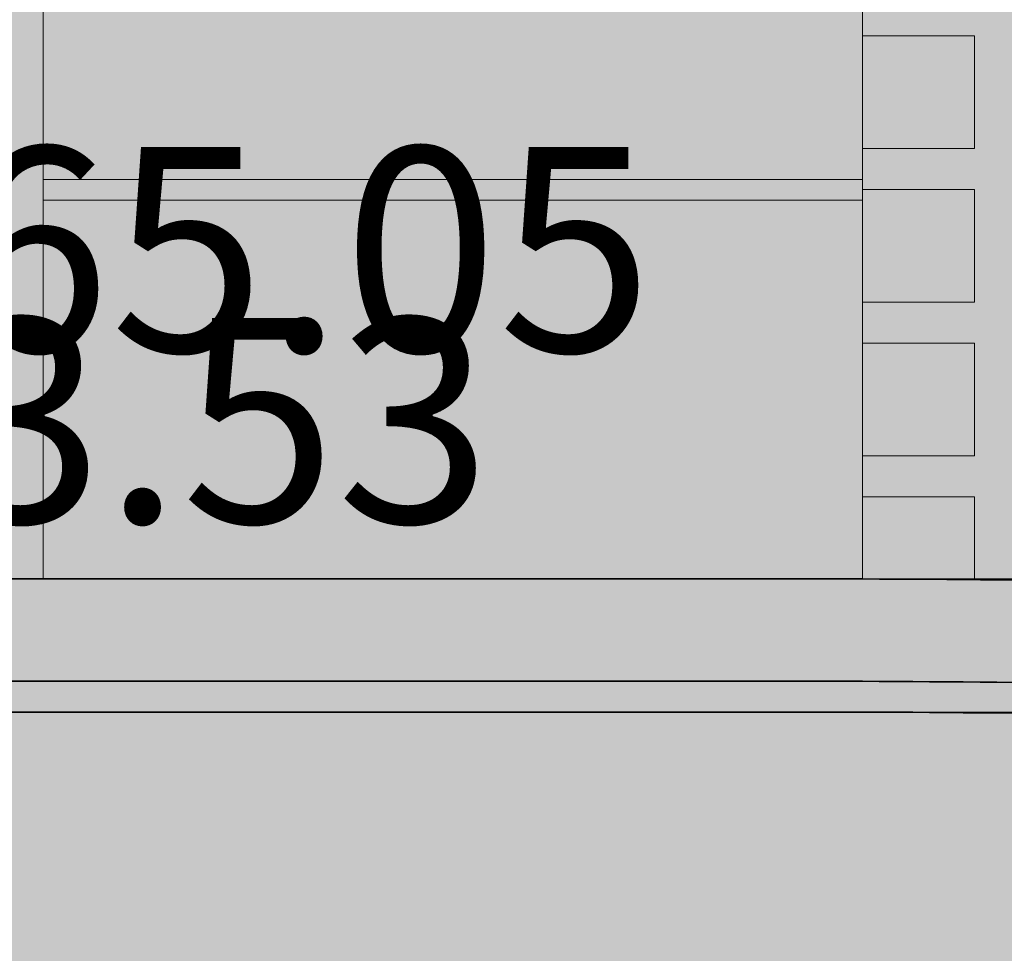
# Model space of a CAD drawing. Units: millimetres. Extents: x 130 to 1021, y 147 to 699.
# Tile 36 of 40: x 550 to 646, y 440 to 532. Entities that reach past the tile are written whole.
import ezdxf

# ---------------------------------------------------------------- set-up
doc = ezdxf.new("R2010")
doc.units = ezdxf.units.MM
doc.header["$MEASUREMENT"] = 0
for name, color, linetype, lineweight in [('A-ANNO-DIMS', 2, 'Continuous', 18), ('A-ELEV', 7, 'Continuous', 35), ('A-ELEV-PATT', 9, 'Continuous', 13), ('A-GLAZ', 4, 'Continuous', 18)]:
    doc.layers.add(name, color=color, linetype=linetype, lineweight=lineweight)
doc.styles.get("Standard").update_dxf_attribs({"font": 'arial.ttf'})
doc.dimstyles.get("Standard").update_dxf_attribs({"dimtxt": 20, "dimasz": 10, "dimexe": 10, "dimexo": 10, "dimgap": 5, "dimtad": 0, "dimtih": 1, "dimtoh": 1, "dimdec": 0, "dimzin": 0, "dimdsep": 46, "dimtxsty": 'Standard', "dimcen": 5, "dimadec": 0, "dimazin": 0, "dimtfac": 1, "dimtdec": 0, "dimtofl": 0, "dimtmove": 0, "dimatfit": 3, "dimfxl": 1, "dimtolj": 1, "dimtzin": 0, "dimarcsym": 0})

# ---------------------------------------------------------------- blocks, each defined once
blk = doc.blocks.new('*D11')
at = {"layer": 'A-ANNO-DIMS', "color": 0, "lineweight": -2, "transparency": 16777216}
for p, q in [((737.374, 648.699), (737.374, 149.739)), ((299.374, 566.947), (299.374, 149.739)), ((309.374, 159.739), (490.857, 159.739)), ((727.374, 159.739), (545.891, 159.739))]:
    blk.add_line(p, q, dxfattribs=at)
at = {"layer": 'A-ANNO-DIMS', "color": 0, "transparency": 16777216}
for points in [[(309.374, 161.406), (309.374, 158.073), (299.374, 159.739)], [(727.374, 161.406), (727.374, 158.073), (737.374, 159.739)]]:
    blk.add_solid(points, dxfattribs=at)
at = {"layer": 'Defpoints', "color": 0, "transparency": 16777216}
for p in [(737.374, 658.699), (299.374, 576.947), (737.374, 159.739)]:
    blk.add_point(p, dxfattribs=at)
at = {"layer": 'A-ANNO-DIMS', "color": 0, "transparency": 16777216, "insert": (518.374, 159.739), "char_height": 20, "attachment_point": 5}
blk.add_mtext('\\A1;438', dxfattribs=at)
blk = doc.blocks.new('*D22')
at = {"layer": 'A-ANNO-DIMS', "color": 0, "lineweight": -2, "transparency": 16777216}
for p, q in [((447.374, 656.947), (447.374, 696.247)), ((466.767, 403.947), (466.767, 696.247)), ((437.374, 686.247), (427.374, 686.247)), ((476.767, 686.247), (486.767, 686.247))]:
    blk.add_line(p, q, dxfattribs=at)
at = {"layer": 'A-ANNO-DIMS', "color": 0, "transparency": 16777216}
for points in [[(437.374, 687.914), (437.374, 684.581), (447.374, 686.247)], [(476.767, 687.914), (476.767, 684.581), (466.767, 686.247)]]:
    blk.add_solid(points, dxfattribs=at)
at = {"layer": 'Defpoints', "color": 0, "transparency": 16777216}
for p in [(466.767, 686.247), (447.374, 646.947), (466.767, 393.947)]:
    blk.add_point(p, dxfattribs=at)
at = {"layer": 'A-ANNO-DIMS', "color": 0, "transparency": 16777216, "insert": (532.34, 686.247), "char_height": 20, "attachment_point": 5}
blk.add_mtext('\\A1;19.393', dxfattribs=at)
blk = doc.blocks.new('*D23')
at = {"layer": 'A-ANNO-DIMS', "color": 0, "lineweight": -2, "transparency": 16777216}
for p, q in [((466.767, 403.947), (466.767, 696.247)), ((475.988, 209.039), (475.988, 696.247)), ((456.767, 686.247), (446.767, 686.247)), ((485.988, 686.247), (495.988, 686.247))]:
    blk.add_line(p, q, dxfattribs=at)
at = {"layer": 'A-ANNO-DIMS', "color": 0, "transparency": 16777216}
for points in [[(456.767, 687.914), (456.767, 684.581), (466.767, 686.247)], [(485.988, 687.914), (485.988, 684.581), (475.988, 686.247)]]:
    blk.add_solid(points, dxfattribs=at)
at = {"layer": 'Defpoints', "color": 0, "transparency": 16777216}
for p in [(475.988, 686.247), (466.767, 393.947), (475.988, 199.039)]:
    blk.add_point(p, dxfattribs=at)
at = {"layer": 'A-ANNO-DIMS', "color": 0, "transparency": 16777216, "insert": (534.631, 686.247), "char_height": 20, "attachment_point": 5}
blk.add_mtext('\\A1;9.222', dxfattribs=at)
blk = doc.blocks.new('*D24')
at = {"layer": 'A-ANNO-DIMS', "color": 0, "lineweight": -2, "transparency": 16777216}
for p, q in [((475.988, 209.039), (475.988, 696.247)), ((487.374, 671.947), (487.374, 696.247)), ((465.988, 686.247), (455.988, 686.247)), ((497.374, 686.247), (507.374, 686.247))]:
    blk.add_line(p, q, dxfattribs=at)
at = {"layer": 'A-ANNO-DIMS', "color": 0, "transparency": 16777216}
for points in [[(465.988, 687.914), (465.988, 684.581), (475.988, 686.247)], [(497.374, 687.914), (497.374, 684.581), (487.374, 686.247)]]:
    blk.add_solid(points, dxfattribs=at)
at = {"layer": 'Defpoints', "color": 0, "transparency": 16777216}
for p in [(487.374, 686.247), (487.374, 661.947), (475.988, 199.039)]:
    blk.add_point(p, dxfattribs=at)
at = {"layer": 'A-ANNO-DIMS', "color": 0, "transparency": 16777216, "insert": (553.022, 686.247), "char_height": 20, "attachment_point": 5}
blk.add_mtext('\\A1;11.385', dxfattribs=at)
blk = doc.blocks.new('*D25')
at = {"layer": 'A-ANNO-DIMS', "color": 0, "lineweight": -2, "transparency": 16777216}
for p, q in [((487.374, 671.947), (487.374, 696.247)), ((494.102, 506.908), (494.102, 696.247)), ((477.374, 686.247), (467.374, 686.247)), ((504.102, 686.247), (514.102, 686.247))]:
    blk.add_line(p, q, dxfattribs=at)
at = {"layer": 'A-ANNO-DIMS', "color": 0, "transparency": 16777216}
for points in [[(477.374, 687.914), (477.374, 684.581), (487.374, 686.247)], [(504.102, 687.914), (504.102, 684.581), (494.102, 686.247)]]:
    blk.add_solid(points, dxfattribs=at)
at = {"layer": 'Defpoints', "color": 0, "transparency": 16777216}
for p in [(494.102, 686.247), (487.374, 661.947), (494.102, 496.908)]:
    blk.add_point(p, dxfattribs=at)
at = {"layer": 'A-ANNO-DIMS', "color": 0, "transparency": 16777216, "insert": (552.922, 686.247), "char_height": 20, "attachment_point": 5}
blk.add_mtext('\\A1;6.728', dxfattribs=at)
blk = doc.blocks.new('*D26')
at = {"layer": 'A-ANNO-DIMS', "color": 0, "lineweight": -2, "transparency": 16777216}
for p, q in [((494.102, 506.908), (494.102, 696.247)), ((502.374, 593.947), (502.374, 696.247)), ((484.102, 686.247), (474.102, 686.247)), ((512.374, 686.247), (522.374, 686.247))]:
    blk.add_line(p, q, dxfattribs=at)
at = {"layer": 'A-ANNO-DIMS', "color": 0, "transparency": 16777216}
for points in [[(484.102, 687.914), (484.102, 684.581), (494.102, 686.247)], [(512.374, 687.914), (512.374, 684.581), (502.374, 686.247)]]:
    blk.add_solid(points, dxfattribs=at)
at = {"layer": 'Defpoints', "color": 0, "transparency": 16777216}
for p in [(502.374, 686.247), (502.374, 583.947), (494.102, 496.908)]:
    blk.add_point(p, dxfattribs=at)
at = {"layer": 'A-ANNO-DIMS', "color": 0, "transparency": 16777216, "insert": (561.03, 686.247), "char_height": 20, "attachment_point": 5}
blk.add_mtext('\\A1;8.272', dxfattribs=at)
blk = doc.blocks.new('*D27')
at = {"layer": 'A-ANNO-DIMS', "color": 0, "lineweight": -2, "transparency": 16777216}
for p, q in [((502.374, 593.947), (502.374, 696.247)), ((544.635, 396.264), (544.635, 696.247)), ((512.374, 686.247), (534.635, 686.247)), ((544.635, 686.247), (554.635, 686.247))]:
    blk.add_line(p, q, dxfattribs=at)
at = {"layer": 'A-ANNO-DIMS', "color": 0, "transparency": 16777216}
for points in [[(512.374, 687.914), (512.374, 684.581), (502.374, 686.247)], [(534.635, 687.914), (534.635, 684.581), (544.635, 686.247)]]:
    blk.add_solid(points, dxfattribs=at)
at = {"layer": 'Defpoints', "color": 0, "transparency": 16777216}
for p in [(544.635, 686.247), (502.374, 583.947), (544.635, 386.264)]:
    blk.add_point(p, dxfattribs=at)
at = {"layer": 'A-ANNO-DIMS', "color": 0, "transparency": 16777216, "insert": (593.776, 686.247), "char_height": 20, "attachment_point": 5}
blk.add_mtext('\\A1;42.26', dxfattribs=at)
blk = doc.blocks.new('*D28')
at = {"layer": 'A-ANNO-DIMS', "color": 0, "lineweight": -2, "transparency": 16777216}
for p, q in [((544.635, 396.264), (544.635, 696.247)), ((552.374, 593.947), (552.374, 696.247)), ((534.635, 686.247), (524.635, 686.247)), ((562.374, 686.247), (572.374, 686.247))]:
    blk.add_line(p, q, dxfattribs=at)
at = {"layer": 'A-ANNO-DIMS', "color": 0, "transparency": 16777216}
for points in [[(534.635, 687.914), (534.635, 684.581), (544.635, 686.247)], [(562.374, 687.914), (562.374, 684.581), (552.374, 686.247)]]:
    blk.add_solid(points, dxfattribs=at)
at = {"layer": 'Defpoints', "color": 0, "transparency": 16777216}
for p in [(552.374, 686.247), (552.374, 583.947), (544.635, 386.264)]:
    blk.add_point(p, dxfattribs=at)
at = {"layer": 'A-ANNO-DIMS', "color": 0, "transparency": 16777216, "insert": (611.057, 686.247), "char_height": 20, "attachment_point": 5}
blk.add_mtext('\\A1;7.738', dxfattribs=at)
blk = doc.blocks.new('*D54')
at = {"layer": 'A-ANNO-DIMS', "color": 0, "lineweight": -2, "transparency": 16777216}
for p, q in [((761.674, 473.947), (761.674, 483.947)), ((497.374, 463.947), (771.674, 463.947)), ((747.374, 403.69), (771.674, 403.69)), ((761.674, 393.69), (761.674, 383.69))]:
    blk.add_line(p, q, dxfattribs=at)
at = {"layer": 'A-ANNO-DIMS', "color": 0, "transparency": 16777216}
for points in [[(760.007, 473.947), (763.34, 473.947), (761.674, 463.947)], [(760.007, 393.69), (763.34, 393.69), (761.674, 403.69)]]:
    blk.add_solid(points, dxfattribs=at)
at = {"layer": 'Defpoints', "color": 0, "transparency": 16777216}
for p in [(487.374, 463.947), (761.674, 463.947), (737.374, 403.69)]:
    blk.add_point(p, dxfattribs=at)
at = {"layer": 'A-ANNO-DIMS', "color": 0, "transparency": 16777216, "insert": (761.674, 433.819), "char_height": 20, "attachment_point": 5}
blk.add_mtext('\\A1;60.26', dxfattribs=at)
blk = doc.blocks.new('*D55')
at = {"layer": 'A-ANNO-DIMS', "color": 0, "lineweight": -2, "transparency": 16777216}
for p, q in [((761.674, 486.947), (761.674, 496.947)), ((761.674, 496.947), (771.674, 496.947)), ((562.374, 476.947), (771.674, 476.947)), ((497.374, 463.947), (771.674, 463.947)), ((761.674, 453.947), (761.674, 443.947))]:
    blk.add_line(p, q, dxfattribs=at)
at = {"layer": 'A-ANNO-DIMS', "color": 0, "transparency": 16777216}
for points in [[(760.007, 486.947), (763.34, 486.947), (761.674, 476.947)], [(760.007, 453.947), (763.34, 453.947), (761.674, 463.947)]]:
    blk.add_solid(points, dxfattribs=at)
at = {"layer": 'Defpoints', "color": 0, "transparency": 16777216}
for p in [(552.374, 476.947), (761.674, 476.947), (487.374, 463.947)]:
    blk.add_point(p, dxfattribs=at)
at = {"layer": 'A-ANNO-DIMS', "color": 0, "transparency": 16777216, "insert": (790.057, 496.947), "char_height": 20, "attachment_point": 5}
blk.add_mtext('\\A1;13', dxfattribs=at)
blk = doc.blocks.new('*D56')
at = {"layer": 'A-ANNO-DIMS', "color": 0, "lineweight": -2, "transparency": 16777216}
for p, q in [((562.374, 583.947), (771.674, 583.947)), ((761.674, 573.947), (761.674, 545.659)), ((761.674, 486.947), (761.674, 515.236)), ((562.374, 476.947), (771.674, 476.947))]:
    blk.add_line(p, q, dxfattribs=at)
at = {"layer": 'A-ANNO-DIMS', "color": 0, "transparency": 16777216}
for points in [[(760.007, 573.947), (763.34, 573.947), (761.674, 583.947)], [(760.007, 486.947), (763.34, 486.947), (761.674, 476.947)]]:
    blk.add_solid(points, dxfattribs=at)
at = {"layer": 'Defpoints', "color": 0, "transparency": 16777216}
for p in [(552.374, 583.947), (761.674, 583.947), (552.374, 476.947)]:
    blk.add_point(p, dxfattribs=at)
at = {"layer": 'A-ANNO-DIMS', "color": 0, "transparency": 16777216, "insert": (761.674, 530.447), "char_height": 20, "attachment_point": 5}
blk.add_mtext('\\A1;107', dxfattribs=at)
blk = doc.blocks.new('*D65')
at = {"layer": 'A-ANNO-DIMS', "color": 0, "lineweight": -2, "transparency": 16777216}
for p, q in [((495.463, 509.127), (472.508, 423.108)), ((505.463, 509.127), (495.463, 509.127)), ((427.374, 248.979), (427.374, 258.979)), ((422.374, 253.979), (432.374, 253.979))]:
    blk.add_line(p, q, dxfattribs=at)
at = {"layer": 'A-ANNO-DIMS', "color": 0, "transparency": 16777216}
blk.add_solid([(470.898, 423.538), (474.118, 422.679), (469.93, 413.447)], dxfattribs=at)
at = {"layer": 'Defpoints', "color": 0, "transparency": 16777216}
for p in [(469.93, 413.447), (427.374, 253.979)]:
    blk.add_point(p, dxfattribs=at)
at = {"layer": 'A-ANNO-DIMS', "color": 0, "transparency": 16777216, "insert": (561.623, 509.127), "char_height": 20, "attachment_point": 5}
blk.add_mtext('\\A1;R165.05', dxfattribs=at)
blk = doc.blocks.new('*D67')
at = {"layer": 'A-ANNO-DIMS', "color": 0, "lineweight": -2, "transparency": 16777216}
for p, q in [((479.756, 492.431), (462.144, 412.223)), ((489.756, 492.431), (479.756, 492.431)), ((427.07, 247.496), (427.07, 257.496)), ((422.07, 252.496), (432.07, 252.496))]:
    blk.add_line(p, q, dxfattribs=at)
at = {"layer": 'A-ANNO-DIMS', "color": 0, "transparency": 16777216}
blk.add_solid([(460.516, 412.58), (463.772, 411.865), (459.999, 402.455)], dxfattribs=at)
at = {"layer": 'Defpoints', "color": 0, "transparency": 16777216}
for p in [(459.999, 402.455), (427.07, 252.496)]:
    blk.add_point(p, dxfattribs=at)
at = {"layer": 'A-ANNO-DIMS', "color": 0, "transparency": 16777216, "insert": (545.841, 492.431), "char_height": 20, "attachment_point": 5}
blk.add_mtext('\\A1;R153.53', dxfattribs=at)
blk = doc.blocks.new('*D69')
at = {"layer": 'A-ANNO-DIMS', "color": 0, "lineweight": -2, "transparency": 16777216}
for p, q in [((507.746, 572.261), (483.091, 501.813)), ((517.746, 572.261), (507.746, 572.261)), ((433.191, 354.23), (433.191, 364.23)), ((428.191, 359.23), (438.191, 359.23))]:
    blk.add_line(p, q, dxfattribs=at)
at = {"layer": 'A-ANNO-DIMS', "color": 0, "transparency": 16777216}
blk.add_solid([(481.518, 502.363), (484.664, 501.262), (479.788, 492.374)], dxfattribs=at)
at = {"layer": 'Defpoints', "color": 0, "transparency": 16777216}
for p in [(479.788, 492.374), (433.191, 359.23)]:
    blk.add_point(p, dxfattribs=at)
at = {"layer": 'A-ANNO-DIMS', "color": 0, "transparency": 16777216, "insert": (573.824, 572.261), "char_height": 20, "attachment_point": 5}
blk.add_mtext('\\A1;R141.06', dxfattribs=at)
blk = doc.blocks.new('*D71')
at = {"layer": 'A-ANNO-DIMS', "color": 0, "lineweight": -2, "transparency": 16777216}
for p, q in [((492.108, 581.609), (472.542, 512.666)), ((502.108, 581.609), (492.108, 581.609)), ((432.65, 367.109), (432.65, 377.109)), ((427.65, 372.109), (437.65, 372.109))]:
    blk.add_line(p, q, dxfattribs=at)
at = {"layer": 'A-ANNO-DIMS', "color": 0, "transparency": 16777216}
blk.add_solid([(470.938, 513.121), (474.145, 512.211), (469.812, 503.046)], dxfattribs=at)
at = {"layer": 'Defpoints', "color": 0, "transparency": 16777216}
for p in [(469.812, 503.046), (432.65, 372.109)]:
    blk.add_point(p, dxfattribs=at)
at = {"layer": 'A-ANNO-DIMS', "color": 0, "transparency": 16777216, "insert": (548.493, 581.609), "char_height": 20, "attachment_point": 5}
blk.add_mtext('\\A1;R136.1', dxfattribs=at)
blk = doc.blocks.new('*D72')
at = {"layer": 'A-ANNO-DIMS', "color": 0, "lineweight": -2, "transparency": 16777216}
for p, q in [((460.658, 573.64), (451.279, 503.49)), ((470.658, 573.64), (460.658, 573.64)), ((432.115, 355.142), (432.115, 365.142)), ((427.115, 360.142), (437.115, 360.142))]:
    blk.add_line(p, q, dxfattribs=at)
at = {"layer": 'A-ANNO-DIMS', "color": 0, "transparency": 16777216}
blk.add_solid([(449.628, 503.711), (452.931, 503.27), (449.954, 493.579)], dxfattribs=at)
at = {"layer": 'Defpoints', "color": 0, "transparency": 16777216}
for p in [(449.954, 493.579), (432.115, 360.142)]:
    blk.add_point(p, dxfattribs=at)
at = {"layer": 'A-ANNO-DIMS', "color": 0, "transparency": 16777216, "insert": (526.64, 573.64), "char_height": 20, "attachment_point": 5}
blk.add_mtext('\\A1;R134.62', dxfattribs=at)

msp = doc.modelspace()

# ---------------------------------------------------------------- hatches: boundary and pattern name
at = {"layer": 'A-ELEV-PATT'}
h = msp.add_hatch(color=256, dxfattribs=at)
h.dxf.hatch_style = 1
h.paths.add_polyline_path([(737.3738, 658.6988, 0.0135961), (632.4019, 661.9473), (607.3738, 661.9473), (487.3738, 661.9473), (487.3738, 649.9473), (607.3738, 649.9473), (632.3794, 649.9473, -0.0136841), (737.3738, 646.6784)])
h.paths.add_polyline_path([(732.3738, 643.9599, 0.0130529), (632.3738, 646.9473), (607.3738, 646.9473), (487.3738, 646.9473), (487.3738, 596.9473), (632.3738, 596.9473, -0.0130529), (732.3738, 593.9599)])
h.paths.add_polyline_path([(737.3738, 593.6732, 0.0137063), (632.3738, 596.9473), (487.3738, 596.9473), (487.3738, 586.9473), (632.355, 586.9473, -0.0137808), (737.3738, 583.6559)])
h.paths.add_polyline_path([(447.3738, 646.9473), (307.3738, 646.9473), (302.3738, 646.9473), (302.3738, 634.9473), (447.3738, 634.9473)])
h.paths.add_polyline_path([(447.3738, 631.9473), (307.3738, 631.9473), (307.3738, 586.9473), (447.3738, 586.9473)])
h.paths.add_polyline_path([(447.3738, 586.9473), (307.3738, 586.9473), (302.3738, 586.9473), (302.3738, 576.9473), (447.3738, 576.9473)])
h.paths.add_polyline_path([(447.3738, 573.9473), (367.3738, 573.9473), (367.3738, 539.9473), (447.3738, 539.9473)])
h.paths.add_polyline_path([(447.3738, 537.9473), (367.3738, 537.9473), (367.3738, 507.9473), (400.392, 507.4253, -0.001728), (401.3281, 507.6451, -0.5220025), (425.6117, 511.0391, -0.0391849), (447.3738, 510.4359), (447.3738, 510.7883)])
h.paths.add_polyline_path([(394.7238, 505.9473), (367.3738, 505.9473), (367.3738, 476.9473, -0.0146512), (375.8501, 480.2159), (376.1506, 499.2266, -0.0355419)])
h.paths.add_polyline_path([(632.3738, 583.9473), (552.3738, 583.9473), (552.3738, 550.9473), (632.3738, 550.9473)])
h.paths.add_polyline_path([(632.3738, 548.9473), (552.3738, 548.9473), (552.3738, 515.9473), (632.3738, 515.9473)])
h.paths.add_polyline_path([(632.3738, 513.9473), (552.3738, 513.9473), (552.3738, 476.9473), (632.3738, 476.9473)])
h.paths.add_polyline_path([(737.3738, 473.6903, 0.0136326), (632.3926, 476.9473), (552.3738, 476.9473), (487.3738, 476.9473), (487.3738, 466.9473), (632.3738, 466.9473, -0.0137063), (737.3738, 463.6732)])
h.paths.add_polyline_path([(732.3738, 460.9552, 0.0130741), (632.3681, 463.9473), (487.3738, 463.9473), (487.3738, 407.735, -0.0032286), (489.3544, 406.9473), (632.3926, 406.9473, -0.0129826), (732.3738, 403.9755)])
h.paths.add_polyline_path([(487.3738, 463.9473, 0.20133), (367.3738, 463.9473), (367.3738, 407.735, -0.1882031), (487.3738, 407.735)])
h.paths.add_polyline_path([(367.3738, 476.9473), (367.3738, 466.9473, -0.2013309), (487.3738, 466.9473), (487.3738, 476.9473, 0.20133)])
h.paths.add_polyline_path([(367.3738, 463.9473), (307.3738, 463.9473), (307.3738, 401.9473), (357.9413, 401.9473), (367.3738, 407.735)])
h.paths.add_polyline_path([(367.3738, 476.9473), (302.3738, 476.9473), (302.3738, 466.9473), (367.3738, 466.9473)])
h.paths.add_polyline_path([(632.8184, 366.9453), (552.3738, 366.9453), (552.3738, 393.9473), (632.8184, 393.9473)])
h.paths.add_polyline_path([(632.8184, 357.2114), (632.8184, 363.9453), (552.3738, 363.9453), (552.3738, 357.2114), (552.3738, 336.9453), (632.8184, 336.9453)])
h.paths.add_polyline_path([(632.8184, 333.9453), (552.3738, 333.9453), (552.3738, 306.9453), (632.8184, 306.9453)])
h.paths.add_polyline_path([(632.8184, 303.9453), (552.3738, 303.9453), (552.3738, 273.9473), (632.355, 273.9473, 0.0000608), (632.8184, 273.9491)])
h.paths.add_polyline_path([(737.3738, 403.6903, 0.0136326), (632.3926, 406.9473), (489.3544, 406.9473, 0.1915481), (367.3738, 407.735), (367.3738, 396.9473, -0.2013309), (487.3738, 396.9473), (632.3738, 396.9473, -0.0137063), (737.3738, 393.6732)])
h.paths.add_polyline_path([(357.9413, 401.9473), (307.3738, 401.9473), (307.3738, 391.9473), (357.9413, 391.9473)])
h.paths.add_polyline_path([(357.9413, 357.2114), (357.9413, 388.9473), (307.3738, 388.9473), (307.3738, 357.2114), (307.3738, 273.9473), (357.9413, 273.9473)])
h.paths.add_polyline_path([(732.3738, 263.93, -0.0130317), (632.3794, 260.9473), (466.7667, 260.9473), (466.7667, 240.9473), (469.8406, 236.978), (469.8406, 221.978), (472.9145, 218.0087), (472.9145, 213.9473), (607.3738, 213.9473), (732.3738, 213.9473)])
h.paths.add_polyline_path([(732.3738, 290.889), (722.479, 290.889), (722.479, 301.889), (732.3738, 301.889), (732.3738, 305.889), (722.479, 305.889), (722.479, 316.889), (732.3738, 316.889), (732.3738, 320.889), (722.479, 320.889), (722.479, 331.889), (732.3738, 331.889), (732.3738, 335.889), (722.479, 335.889), (722.479, 346.889), (732.3738, 346.889), (732.3738, 350.889), (722.479, 350.889), (722.479, 361.889), (732.3738, 361.889), (732.3738, 365.889), (722.479, 365.889), (722.479, 376.889), (732.3738, 376.889), (732.3738, 380.889), (722.479, 380.889), (722.479, 391.4848, 0.0005233), (718.479, 391.6843), (718.479, 380.889), (707.479, 380.889), (707.479, 392.1896, 0.0005231), (703.479, 392.3576), (703.479, 380.889), (692.479, 380.889), (692.479, 392.7765, 0.0005229), (688.479, 392.9131), (688.479, 380.889), (677.479, 380.889), (677.479, 393.2456, 0.0005228), (673.479, 393.3508), (673.479, 380.889), (662.479, 380.889), (662.479, 393.597, 0.0005227), (658.479, 393.6709), (658.479, 380.889), (647.479, 380.889), (647.479, 393.8308, 0.0005226), (643.479, 393.8732), (643.479, 380.889), (632.8184, 380.889), (632.8184, 376.889), (643.479, 376.889), (643.479, 365.889), (632.8184, 365.889), (632.8184, 361.889), (643.479, 361.889), (643.479, 350.889), (632.8184, 350.889), (632.8184, 346.889), (643.479, 346.889), (643.479, 335.889), (632.8184, 335.889), (632.8184, 331.889), (643.479, 331.889), (643.479, 320.889), (632.8184, 320.889), (632.8184, 316.889), (643.479, 316.889), (643.479, 305.889), (632.8184, 305.889), (632.8184, 301.889), (643.479, 301.889), (643.479, 290.889), (632.8184, 290.889), (632.8184, 286.889), (643.479, 286.889), (643.479, 274.0217, 0.0005246), (647.479, 274.0643), (647.479, 286.889), (658.479, 286.889), (658.479, 274.2248, 0.0005246), (662.479, 274.2989), (662.479, 286.889), (673.479, 286.889), (673.479, 274.546, 0.0005247), (677.479, 274.6516), (677.479, 286.889), (688.479, 286.889), (688.479, 274.9853, 0.0005248), (692.479, 275.1224), (692.479, 286.889), (703.479, 286.889), (703.479, 275.5429, 0.000525), (707.479, 275.7115), (707.479, 286.889), (718.479, 286.889), (718.479, 276.2187, 0.0005252), (722.479, 276.4189), (722.479, 286.889), (732.3738, 286.889)])
h.paths.add_polyline_path([(718.479, 290.889), (707.479, 290.889), (707.479, 301.889), (718.479, 301.889)], flags=16)
h.paths.add_polyline_path([(703.479, 290.889), (692.479, 290.889), (692.479, 301.889), (703.479, 301.889)], flags=16)
h.paths.add_polyline_path([(718.479, 305.889), (707.479, 305.889), (707.479, 316.889), (718.479, 316.889)], flags=16)
h.paths.add_polyline_path([(703.479, 305.889), (692.479, 305.889), (692.479, 316.889), (703.479, 316.889)], flags=16)
h.paths.add_polyline_path([(688.479, 290.889), (677.479, 290.889), (677.479, 301.889), (688.479, 301.889)], flags=16)
h.paths.add_polyline_path([(718.479, 320.889), (707.479, 320.889), (707.479, 331.889), (718.479, 331.889)], flags=16)
h.paths.add_polyline_path([(688.479, 305.889), (677.479, 305.889), (677.479, 316.889), (688.479, 316.889)], flags=16)
h.paths.add_polyline_path([(703.479, 320.889), (692.479, 320.889), (692.479, 331.889), (703.479, 331.889)], flags=16)
h.paths.add_polyline_path([(688.479, 320.889), (677.479, 320.889), (677.479, 331.889), (688.479, 331.889)], flags=16)
h.paths.add_polyline_path([(673.479, 290.889), (662.479, 290.889), (662.479, 301.889), (673.479, 301.889)], flags=16)
h.paths.add_polyline_path([(718.479, 335.889), (707.479, 335.889), (707.479, 346.889), (718.479, 346.889)], flags=16)
h.paths.add_polyline_path([(673.479, 305.889), (662.479, 305.889), (662.479, 316.889), (673.479, 316.889)], flags=16)
h.paths.add_polyline_path([(703.479, 335.889), (692.479, 335.889), (692.479, 346.889), (703.479, 346.889)], flags=16)
h.paths.add_polyline_path([(673.479, 320.889), (662.479, 320.889), (662.479, 331.889), (673.479, 331.889)], flags=16)
h.paths.add_polyline_path([(688.479, 335.889), (677.479, 335.889), (677.479, 346.889), (688.479, 346.889)], flags=16)
h.paths.add_polyline_path([(658.479, 290.889), (647.479, 290.889), (647.479, 301.889), (658.479, 301.889)], flags=16)
h.paths.add_polyline_path([(718.479, 350.889), (707.479, 350.889), (707.479, 361.889), (718.479, 361.889)], flags=16)
h.paths.add_polyline_path([(658.479, 305.889), (647.479, 305.889), (647.479, 316.889), (658.479, 316.889)], flags=16)
h.paths.add_polyline_path([(703.479, 350.889), (692.479, 350.889), (692.479, 361.889), (703.479, 361.889)], flags=16)
h.paths.add_polyline_path([(673.479, 335.889), (662.479, 335.889), (662.479, 346.889), (673.479, 346.889)], flags=16)
h.paths.add_polyline_path([(658.479, 320.889), (647.479, 320.889), (647.479, 331.889), (658.479, 331.889)], flags=16)
h.paths.add_polyline_path([(688.479, 350.889), (677.479, 350.889), (677.479, 361.889), (688.479, 361.889)], flags=16)
h.paths.add_polyline_path([(718.479, 365.889), (707.479, 365.889), (707.479, 376.889), (718.479, 376.889)], flags=16)
h.paths.add_polyline_path([(658.479, 335.889), (647.479, 335.889), (647.479, 346.889), (658.479, 346.889)], flags=16)
h.paths.add_polyline_path([(673.479, 350.889), (662.479, 350.889), (662.479, 361.889), (673.479, 361.889)], flags=16)
h.paths.add_polyline_path([(703.479, 365.889), (692.479, 365.889), (692.479, 376.889), (703.479, 376.889)], flags=16)
h.paths.add_polyline_path([(688.479, 365.889), (677.479, 365.889), (677.479, 376.889), (688.479, 376.889)], flags=16)
h.paths.add_polyline_path([(658.479, 350.889), (647.479, 350.889), (647.479, 361.889), (658.479, 361.889)], flags=16)
h.paths.add_polyline_path([(673.479, 365.889), (662.479, 365.889), (662.479, 376.889), (673.479, 376.889)], flags=16)
h.paths.add_polyline_path([(658.479, 365.889), (647.479, 365.889), (647.479, 376.889), (658.479, 376.889)], flags=16)
h.paths.add_polyline_path([(732.3738, 503.9786), (722.3392, 503.9786), (722.3392, 514.9786), (732.3738, 514.9786), (732.3738, 518.9786), (722.3392, 518.9786), (722.3392, 529.9786), (732.3738, 529.9786), (732.3738, 533.9786), (722.3392, 533.9786), (722.3392, 544.9786), (732.3738, 544.9786), (732.3738, 546.9473), (732.3738, 548.9786), (722.3392, 548.9786), (722.3392, 559.9786), (732.3738, 559.9786), (732.3738, 563.9786), (722.3392, 563.9786), (722.3392, 574.9786), (732.3738, 574.9786), (732.3738, 578.9786), (722.3392, 578.9786), (722.3392, 581.4789, 0.000526), (718.3392, 581.6791), (718.3392, 578.9786), (707.3392, 578.9786), (707.3392, 582.1863, 0.0005258), (703.3392, 582.355), (703.3392, 578.9786), (692.3392, 578.9786), (692.3392, 582.7752, 0.0005257), (688.3392, 582.9123), (688.3392, 578.9786), (677.3392, 578.9786), (677.3392, 583.2457, 0.0005255), (673.3392, 583.3512), (673.3392, 578.9786), (662.3392, 578.9786), (662.3392, 583.5978, 0.0005254), (658.3392, 583.6718), (658.3392, 578.9786), (647.3392, 578.9786), (647.3392, 583.8317, 0.0005254), (643.3392, 583.8741), (643.3392, 578.9786), (632.3738, 578.9786), (632.3738, 574.9786), (643.3392, 574.9786), (643.3392, 563.9786), (632.3738, 563.9786), (632.3738, 559.9786), (643.3392, 559.9786), (643.3392, 548.9786), (632.3738, 548.9786), (632.3738, 544.9786), (643.3392, 544.9786), (643.3392, 533.9786), (632.3738, 533.9786), (632.3738, 529.9786), (643.3392, 529.9786), (643.3392, 518.9786), (632.3738, 518.9786), (632.3738, 515.9473), (632.3738, 514.9786), (643.3392, 514.9786), (643.3392, 503.9786), (632.3738, 503.9786), (632.3738, 499.9786), (643.3392, 499.9786), (643.3392, 488.9786), (632.3738, 488.9786), (632.3738, 484.9786), (643.3392, 484.9786), (643.3392, 476.8751, -0.0005191), (647.3392, 476.8332), (647.3392, 484.9786), (658.3392, 484.9786), (658.3392, 476.6752, -0.0005192), (662.3392, 476.6022), (662.3392, 484.9786), (673.3392, 484.9786), (673.3392, 476.3585, -0.0005193), (677.3392, 476.2543), (677.3392, 484.9786), (688.3392, 484.9786), (688.3392, 475.9248, -0.0005194), (692.3392, 475.7894), (692.3392, 484.9786), (703.3392, 484.9786), (703.3392, 475.3741, -0.0005195), (707.3392, 475.2075), (707.3392, 484.9786), (718.3392, 484.9786), (718.3392, 474.7064, -0.0005197), (722.3392, 474.5086), (722.3392, 484.9786), (732.3738, 484.9786), (732.3738, 488.9786), (722.3392, 488.9786), (722.3392, 499.9786), (732.3738, 499.9786)])
h.paths.add_polyline_path([(718.3392, 503.9786), (707.3392, 503.9786), (707.3392, 514.9786), (718.3392, 514.9786)], flags=16)
h.paths.add_polyline_path([(718.3392, 499.9786), (718.3392, 488.9786), (707.3392, 488.9786), (707.3392, 499.9786)], flags=16)
h.paths.add_polyline_path([(718.3392, 518.9786), (707.3392, 518.9786), (707.3392, 529.9786), (718.3392, 529.9786)], flags=16)
h.paths.add_polyline_path([(703.3392, 503.9786), (692.3392, 503.9786), (692.3392, 514.9786), (703.3392, 514.9786)], flags=16)
h.paths.add_polyline_path([(703.3392, 499.9786), (703.3392, 488.9786), (692.3392, 488.9786), (692.3392, 499.9786)], flags=16)
h.paths.add_polyline_path([(703.3392, 518.9786), (692.3392, 518.9786), (692.3392, 529.9786), (703.3392, 529.9786)], flags=16)
h.paths.add_polyline_path([(718.3392, 533.9786), (707.3392, 533.9786), (707.3392, 544.9786), (718.3392, 544.9786)], flags=16)
h.paths.add_polyline_path([(688.3392, 503.9786), (677.3392, 503.9786), (677.3392, 514.9786), (688.3392, 514.9786)], flags=16)
h.paths.add_polyline_path([(688.3392, 499.9786), (688.3392, 488.9786), (677.3392, 488.9786), (677.3392, 499.9786)], flags=16)
h.paths.add_polyline_path([(703.3392, 533.9786), (692.3392, 533.9786), (692.3392, 544.9786), (703.3392, 544.9786)], flags=16)
h.paths.add_polyline_path([(688.3392, 518.9786), (677.3392, 518.9786), (677.3392, 529.9786), (688.3392, 529.9786)], flags=16)
h.paths.add_polyline_path([(688.3392, 533.9786), (677.3392, 533.9786), (677.3392, 544.9786), (688.3392, 544.9786)], flags=16)
h.paths.add_polyline_path([(718.3392, 548.9786), (707.3392, 548.9786), (707.3392, 559.9786), (718.3392, 559.9786)], flags=16)
h.paths.add_polyline_path([(673.3392, 503.9786), (662.3392, 503.9786), (662.3392, 514.9786), (673.3392, 514.9786)], flags=16)
h.paths.add_polyline_path([(673.3392, 499.9786), (673.3392, 488.9786), (662.3392, 488.9786), (662.3392, 499.9786)], flags=16)
h.paths.add_polyline_path([(703.3392, 548.9786), (692.3392, 548.9786), (692.3392, 559.9786), (703.3392, 559.9786)], flags=16)
h.paths.add_polyline_path([(673.3392, 518.9786), (662.3392, 518.9786), (662.3392, 529.9786), (673.3392, 529.9786)], flags=16)
h.paths.add_polyline_path([(688.3392, 548.9786), (677.3392, 548.9786), (677.3392, 559.9786), (688.3392, 559.9786)], flags=16)
h.paths.add_polyline_path([(673.3392, 533.9786), (662.3392, 533.9786), (662.3392, 544.9786), (673.3392, 544.9786)], flags=16)
h.paths.add_polyline_path([(718.3392, 563.9786), (707.3392, 563.9786), (707.3392, 574.9786), (718.3392, 574.9786)], flags=16)
h.paths.add_polyline_path([(658.3392, 503.9786), (647.3392, 503.9786), (647.3392, 514.9786), (658.3392, 514.9786)], flags=16)
h.paths.add_polyline_path([(658.3392, 499.9786), (658.3392, 488.9786), (647.3392, 488.9786), (647.3392, 499.9786)], flags=16)
h.paths.add_polyline_path([(703.3392, 563.9786), (692.3392, 563.9786), (692.3392, 574.9786), (703.3392, 574.9786)], flags=16)
h.paths.add_polyline_path([(658.3392, 518.9786), (647.3392, 518.9786), (647.3392, 529.9786), (658.3392, 529.9786)], flags=16)
h.paths.add_polyline_path([(673.3392, 548.9786), (662.3392, 548.9786), (662.3392, 559.9786), (673.3392, 559.9786)], flags=16)
h.paths.add_polyline_path([(688.3392, 563.9786), (677.3392, 563.9786), (677.3392, 574.9786), (688.3392, 574.9786)], flags=16)
h.paths.add_polyline_path([(658.3392, 533.9786), (647.3392, 533.9786), (647.3392, 544.9786), (658.3392, 544.9786)], flags=16)
h.paths.add_polyline_path([(673.3392, 563.9786), (662.3392, 563.9786), (662.3392, 574.9786), (673.3392, 574.9786)], flags=16)
h.paths.add_polyline_path([(658.3392, 548.9786), (647.3392, 548.9786), (647.3392, 559.9786), (658.3392, 559.9786)], flags=16)
h.paths.add_polyline_path([(658.3392, 563.9786), (647.3392, 563.9786), (647.3392, 574.9786), (658.3392, 574.9786)], flags=16)
h = msp.add_hatch(color=256, dxfattribs=at)
h.dxf.hatch_style = 1
h.paths.add_polyline_path([(447.3738, 576.9473), (302.3738, 576.9473), (302.3738, 573.9473), (447.3738, 573.9473)])
h.paths.add_polyline_path([(487.3738, 583.9473), (487.3738, 586.9473), (447.3738, 576.9473), (447.3738, 573.9473)])
h.paths.add_polyline_path([(632.355, 586.9473), (487.3738, 586.9473), (487.3738, 583.9473), (632.3738, 583.9473), (632.3738, 583.9472, -0.0138), (737.3738, 580.6507), (737.3738, 583.6559, 0.0137808)])
h.paths.add_polyline_path([(367.3738, 466.9473), (302.3738, 466.9473), (302.3738, 463.9473), (367.3738, 463.9473)])
h.paths.add_polyline_path([(487.3738, 463.9473), (487.3738, 466.9473, 0.2013309), (367.3738, 466.9473), (367.3738, 463.9473, -0.20133)])
h.paths.add_polyline_path([(632.3738, 466.9473), (487.3738, 466.9473), (487.3738, 463.9473), (632.3681, 463.9473, -0.0137285), (737.3738, 460.6681), (737.3738, 463.6732, 0.0137063)])
h.paths.add_polyline_path([(632.3738, 396.9473), (487.3738, 396.9473, 0.2013309), (367.3738, 396.9473), (367.3738, 393.9473, -0.2023717), (486.7667, 393.9473), (632.3681, 393.9473, -0.0137285), (737.3738, 390.6681), (737.3738, 393.6732, 0.0137063)])
h.paths.add_polyline_path([(357.9413, 391.9473), (307.3738, 391.9473), (307.3738, 388.9473), (357.9413, 388.9473)])
h.paths.add_polyline_path([(367.3738, 393.9473), (367.3738, 396.9473), (357.9413, 391.924), (357.9413, 388.9473), (358.058, 388.9473)])
h.paths.add_polyline_path([(737.3738, 264.2162), (737.3738, 267.2214, -0.0137063), (632.3738, 263.9473), (463.7667, 263.9473), (466.7667, 260.9473), (632.3794, 260.9473, 0.0136841)])
h.paths.add_polyline_path([(463.7667, 263.9473), (447.3738, 263.9473), (450.3738, 260.9473), (466.7667, 260.9473)])
h.paths.add_polyline_path([(447.3738, 263.9473), (432.3738, 263.9473), (432.3738, 260.9473), (450.3738, 260.9473)])
h.paths.add_polyline_path([(382.3738, 263.9473), (357.9413, 263.9473), (357.9413, 260.9473), (382.3738, 260.9473)])
h.paths.add_polyline_path([(357.9413, 263.9473), (307.3738, 263.9473), (307.3738, 260.9473), (357.9413, 260.9473)])
msp.add_hatch(color=256, dxfattribs=at).paths.add_polyline_path([(502.3738, 583.9473), (502.3738, 577.3739), (547.7773, 577.3739), (547.7773, 481.7432), (502.3738, 481.7432), (502.3738, 476.9473), (552.3738, 476.9473), (552.3738, 583.9473)])
h = msp.add_hatch(color=256, dxfattribs=at)
h.set_gradient(color1=(122, 175, 223), color2=(76, 153, 95))
h.paths.add_polyline_path([(632.3738, 484.9786), (632.3738, 476.9474, -0.001423), (643.3392, 476.8751), (643.3392, 484.9786)])
h.paths.add_polyline_path([(647.3392, 476.8332, -0.0014276), (658.3392, 476.6752), (658.3392, 484.9786), (647.3392, 484.9786)])
h.paths.add_polyline_path([(673.3392, 484.9786), (662.3392, 484.9786), (662.3392, 476.6022, -0.0014278), (673.3392, 476.3585)])
h.paths.add_polyline_path([(688.3392, 475.9248), (688.3392, 484.9786), (677.3392, 484.9786), (677.3392, 476.2543, -0.0014281)])
h.paths.add_polyline_path([(692.3392, 475.7894, -0.0014285), (703.3392, 475.3741), (703.3392, 484.9786), (692.3392, 484.9786)])
h.paths.add_polyline_path([(718.3392, 474.7064), (718.3392, 484.9786), (707.3392, 484.9786), (707.3392, 475.2075, -0.001429)])
h.paths.add_polyline_path([(722.3392, 474.5086, -0.001304), (732.3738, 473.9755), (732.3738, 484.9786), (722.3392, 484.9786)])
h.paths.add_polyline_path([(722.3392, 488.9786), (732.3738, 488.9786), (732.3738, 499.9786), (722.3392, 499.9786)])
h.paths.add_polyline_path([(707.3392, 499.9786), (707.3392, 488.9786), (718.3392, 488.9786), (718.3392, 499.9786)])
h.paths.add_polyline_path([(703.3392, 499.9786), (692.3392, 499.9786), (692.3392, 488.9786), (703.3392, 488.9786)])
h.paths.add_polyline_path([(688.3392, 499.9786), (677.3392, 499.9786), (677.3392, 488.9786), (688.3392, 488.9786)])
h.paths.add_polyline_path([(673.3392, 499.9786), (662.3392, 499.9786), (662.3392, 488.9786), (673.3392, 488.9786)])
h.paths.add_polyline_path([(658.3392, 499.9786), (647.3392, 499.9786), (647.3392, 488.9786), (658.3392, 488.9786)])
h.paths.add_polyline_path([(643.3392, 499.9786), (632.3738, 499.9786), (632.3738, 488.9786), (643.3392, 488.9786)])
h.paths.add_polyline_path([(643.3392, 514.9786), (632.3738, 514.9786), (632.3738, 503.9786), (643.3392, 503.9786)])
h.paths.add_polyline_path([(647.3392, 503.9786), (658.3392, 503.9786), (658.3392, 514.9786), (647.3392, 514.9786)])
h.paths.add_polyline_path([(673.3392, 514.9786), (662.3392, 514.9786), (662.3392, 503.9786), (673.3392, 503.9786)])
h.paths.add_polyline_path([(688.3392, 503.9786), (688.3392, 514.9786), (677.3392, 514.9786), (677.3392, 503.9786)])
h.paths.add_polyline_path([(692.3392, 503.9786), (703.3392, 503.9786), (703.3392, 514.9786), (692.3392, 514.9786)])
h.paths.add_polyline_path([(718.3392, 503.9786), (718.3392, 514.9786), (707.3392, 514.9786), (707.3392, 503.9786)])
h.paths.add_polyline_path([(732.3738, 503.9786), (732.3738, 514.9786), (722.3392, 514.9786), (722.3392, 503.9786)])
h.paths.add_polyline_path([(732.3738, 529.9786), (722.3392, 529.9786), (722.3392, 518.9786), (732.3738, 518.9786)])
h.paths.add_polyline_path([(707.3392, 518.9786), (718.3392, 518.9786), (718.3392, 529.9786), (707.3392, 529.9786)])
h.paths.add_polyline_path([(692.3392, 518.9786), (703.3392, 518.9786), (703.3392, 529.9786), (692.3392, 529.9786)])
h.paths.add_polyline_path([(688.3392, 529.9786), (677.3392, 529.9786), (677.3392, 518.9786), (688.3392, 518.9786)])
h.paths.add_polyline_path([(673.3392, 518.9786), (673.3392, 529.9786), (662.3392, 529.9786), (662.3392, 518.9786)])
h.paths.add_polyline_path([(658.3392, 529.9786), (647.3392, 529.9786), (647.3392, 518.9786), (658.3392, 518.9786)])
h.paths.add_polyline_path([(632.3738, 529.9786), (632.3738, 518.9786), (643.3392, 518.9786), (643.3392, 529.9786)])
h.paths.add_polyline_path([(643.3392, 533.9786), (643.3392, 544.9786), (632.3738, 544.9786), (632.3738, 533.9786)])
h.paths.add_polyline_path([(647.3392, 533.9786), (658.3392, 533.9786), (658.3392, 544.9786), (647.3392, 544.9786)])
h.paths.add_polyline_path([(662.3392, 533.9786), (673.3392, 533.9786), (673.3392, 544.9786), (662.3392, 544.9786)])
h.paths.add_polyline_path([(677.3392, 533.9786), (688.3392, 533.9786), (688.3392, 544.9786), (677.3392, 544.9786)])
h.paths.add_polyline_path([(692.3392, 533.9786), (703.3392, 533.9786), (703.3392, 544.9786), (692.3392, 544.9786)])
h.paths.add_polyline_path([(707.3392, 533.9786), (718.3392, 533.9786), (718.3392, 544.9786), (707.3392, 544.9786)])
h.paths.add_polyline_path([(722.3392, 533.9786), (732.3738, 533.9786), (732.3738, 544.9786), (722.3392, 544.9786)])
h.paths.add_polyline_path([(632.3738, 559.9786), (632.3738, 548.9786), (643.3392, 548.9786), (643.3392, 559.9786)])
h.paths.add_polyline_path([(632.3738, 574.9786), (632.3738, 563.9786), (643.3392, 563.9786), (643.3392, 574.9786)])
h.paths.add_polyline_path([(632.3738, 583.9472), (632.3738, 578.9786), (643.3392, 578.9786), (643.3392, 583.8741, 0.0014402)])
h.paths.add_polyline_path([(647.3392, 583.8317), (647.3392, 578.9786), (658.3392, 578.9786), (658.3392, 583.6718, 0.0014449)])
h.paths.add_polyline_path([(647.3392, 574.9786), (647.3392, 563.9786), (658.3392, 563.9786), (658.3392, 574.9786)])
h.paths.add_polyline_path([(647.3392, 559.9786), (647.3392, 548.9786), (658.3392, 548.9786), (658.3392, 559.9786)])
h.paths.add_polyline_path([(662.3392, 559.9786), (662.3392, 548.9786), (673.3392, 548.9786), (673.3392, 559.9786)])
h.paths.add_polyline_path([(673.3392, 574.9786), (662.3392, 574.9786), (662.3392, 563.9786), (673.3392, 563.9786)])
h.paths.add_polyline_path([(662.3392, 583.5978), (662.3392, 578.9786), (673.3392, 578.9786), (673.3392, 583.3512, 0.0014451)])
h.paths.add_polyline_path([(688.3392, 578.9786), (688.3392, 582.9123, 0.0014454), (677.3392, 583.2457), (677.3392, 578.9786)])
h.paths.add_polyline_path([(677.3392, 574.9786), (677.3392, 563.9786), (688.3392, 563.9786), (688.3392, 574.9786)])
h.paths.add_polyline_path([(677.3392, 559.9786), (677.3392, 548.9786), (688.3392, 548.9786), (688.3392, 559.9786)])
h.paths.add_polyline_path([(703.3392, 559.9786), (692.3392, 559.9786), (692.3392, 548.9786), (703.3392, 548.9786)])
h.paths.add_polyline_path([(707.3392, 548.9786), (718.3392, 548.9786), (718.3392, 559.9786), (707.3392, 559.9786)])
h.paths.add_polyline_path([(722.3392, 548.9786), (732.3738, 548.9786), (732.3738, 559.9786), (722.3392, 559.9786)])
h.paths.add_polyline_path([(732.3738, 563.9786), (732.3738, 574.9786), (722.3392, 574.9786), (722.3392, 563.9786)])
h.paths.add_polyline_path([(707.3392, 563.9786), (718.3392, 563.9786), (718.3392, 574.9786), (707.3392, 574.9786)])
h.paths.add_polyline_path([(692.3392, 563.9786), (703.3392, 563.9786), (703.3392, 574.9786), (692.3392, 574.9786)])
h.paths.add_polyline_path([(703.3392, 578.9786), (703.3392, 582.355, 0.0014458), (692.3392, 582.7752), (692.3392, 578.9786)])
h.paths.add_polyline_path([(718.3392, 581.6791, 0.0014463), (707.3392, 582.1863), (707.3392, 578.9786), (718.3392, 578.9786)])
h.paths.add_polyline_path([(732.3738, 578.9786), (732.3738, 580.9394, 0.0013198), (722.3392, 581.4789), (722.3392, 578.9786)])
h = msp.add_hatch(color=256, dxfattribs=at)
h.dxf.hatch_style = 1
h.paths.add_polyline_path([(447.3738, 537.9473), (447.3738, 539.9473), (367.3738, 539.9473), (367.3738, 537.9473)])
h.paths.add_polyline_path([(394.7238, 505.9473, -0.0105284), (400.392, 507.4253), (367.3738, 507.9473), (367.3738, 505.9473)])
h.paths.add_polyline_path([(547.7773, 546.9473), (547.7773, 548.9473), (502.3738, 548.9473), (502.3738, 546.9473)])
h.paths.add_polyline_path([(632.3738, 548.9473), (632.3738, 550.9473), (552.3738, 550.9473), (552.3738, 548.9473)])
h.paths.add_polyline_path([(632.3738, 513.9473), (632.3738, 515.9473), (552.3738, 515.9473), (552.3738, 513.9473)])
h.paths.add_polyline_path([(544.6354, 360.9453), (544.6354, 363.9453), (486.7667, 363.9454), (486.7667, 360.9454)])
h.paths.add_polyline_path([(632.8184, 363.9453), (632.8184, 366.9453), (552.3738, 366.9453), (552.3738, 363.9453)])
h.paths.add_polyline_path([(632.8184, 333.9453), (632.8184, 336.9453), (552.3738, 336.9453), (552.3738, 333.9453)])
h.paths.add_polyline_path([(552.3738, 306.9453), (552.3738, 303.9453), (632.8184, 303.9453), (632.8184, 306.9453)])

# ---------------------------------------------------------------- linework, layer by layer
at = {"layer": 'A-ELEV'}
for p, q in [((632.3738, 476.9473), (487.3738, 476.9473)), ((632.3738, 466.9473), (487.3738, 466.9473)), ((632.3738, 463.9473), (487.3738, 463.9473))]:
    msp.add_line(p, q, dxfattribs=at)
for radius, start in [(1926.4697, 86.6609152), (1916.4697, 86.6434721), (1913.4697, 86.6382036)]:
    msp.add_arc((625.1665, -1449.5089), radius, start, 89.784526, dxfattribs=at)
at = {"layer": 'A-GLAZ'}
for p, q in [((552.3738, 583.9473), (552.3738, 476.9473)), ((632.3738, 476.9473), (632.3738, 583.9473)), ((632.3738, 529.9786), (643.3392, 529.9786)), ((643.3392, 518.9786), (643.3392, 529.9786)), ((632.3738, 518.9786), (643.3392, 518.9786)), ((632.3738, 515.9473), (552.3738, 515.9473)), ((632.3738, 514.9786), (643.3392, 514.9786)), ((643.3392, 503.9786), (643.3392, 514.9786)), ((632.3738, 513.9473), (552.3738, 513.9473)), ((632.3738, 503.9786), (643.3392, 503.9786)), ((632.3738, 499.9786), (643.3392, 499.9786)), ((643.3392, 488.9786), (643.3392, 499.9786)), ((632.3738, 488.9786), (643.3392, 488.9786)), ((632.3738, 484.9786), (643.3392, 484.9786)), ((643.3392, 476.8751), (643.3392, 484.9786))]:
    msp.add_line(p, q, dxfattribs=at)

# ---------------------------------------------------------------- dimensions: what is measured, and where the dimension line sits
at = {"layer": 'A-ANNO-DIMS'}
for base, p1, p2, override, picture, middle in [((466.7667, 686.2473), (447.3738, 646.9473), (466.7667, 393.9473), {"dimdec": 3, "dimlfac": 1, "dimrnd": 0, "dimzin": 0, "dimdsep": 46, "dimlunit": 2}, '*D22', (532.3397, 686.2473)), ((475.9885, 686.2473), (466.7667, 393.9473), (475.9885, 199.0395), {"dimdec": 3, "dimlfac": 1, "dimrnd": 0, "dimzin": 0, "dimdsep": 46, "dimlunit": 2}, '*D23', (534.631, 686.2473)), ((487.3738, 686.2473), (475.9885, 199.0395), (487.3738, 661.9473), {"dimdec": 3, "dimlfac": 1, "dimrnd": 0, "dimzin": 0, "dimdsep": 46, "dimlunit": 2}, '*D24', (553.0218, 686.2473)), ((494.10227, 686.2473), (487.37378, 661.9473), (494.10227, 496.90803), {"dimdec": 3, "dimlfac": 1, "dimrnd": 0, "dimzin": 0, "dimdsep": 46, "dimlunit": 2}, '*D25', (552.92219, 686.2473)), ((502.37378, 686.2473), (494.10227, 496.90803), (502.37378, 583.9473), {"dimdec": 3, "dimlfac": 1, "dimrnd": 0, "dimzin": 0, "dimdsep": 46, "dimlunit": 2}, '*D26', (561.02999, 686.2473)), ((544.6354, 686.2473), (502.3738, 583.9473), (544.6354, 386.2639), {"dimdec": 2, "dimlfac": 1, "dimrnd": 0, "dimzin": 0, "dimdsep": 46, "dimlunit": 2}, '*D27', (593.776, 686.2473)), ((552.3738, 686.2473), (544.6354, 386.2639), (552.3738, 583.9473), {"dimdec": 3, "dimlfac": 1, "dimrnd": 0, "dimzin": 0, "dimdsep": 46, "dimlunit": 2}, '*D28', (611.0573, 686.2473)), ((737.3738, 159.7395), (299.3738, 576.9473), (737.3738, 658.6988), {"dimdec": 0, "dimlfac": 1, "dimrnd": 0, "dimzin": 0, "dimdsep": 46, "dimlunit": 2}, '*D11', (518.3738, 159.7395))]:
    dim = msp.add_linear_dim(base=base, p1=p1, p2=p2, dimstyle='Standard', override=override, dxfattribs=at)
    dim.commit()
    dim.dimension.update_dxf_attribs({"geometry": picture, "text_midpoint": middle})
for center, mpoint, override, picture, middle in [((432.6505, 372.1087), (469.8116, 503.0461), {"dimdec": 1, "dimlfac": 1, "dimrnd": 0, "dimzin": 0, "dimdsep": 46, "dimlunit": 2}, '*D71', (548.493, 581.6085)), ((432.115, 360.1423), (449.9544, 493.5786), {"dimdec": 2, "dimlfac": 1, "dimrnd": 0, "dimzin": 0, "dimdsep": 46, "dimlunit": 2}, '*D72', (526.6403, 573.6404)), ((433.1906, 359.2304), (479.788, 492.3743), {"dimdec": 2, "dimlfac": 1, "dimrnd": 0, "dimzin": 0, "dimdsep": 46, "dimlunit": 2}, '*D69', (573.8242, 572.2606)), ((427.3738, 253.9788), (469.9297, 413.4465), {"dimdec": 2, "dimlfac": 1, "dimrnd": 0, "dimzin": 0, "dimdsep": 46, "dimlunit": 2}, '*D65', (561.6228, 509.1272)), ((427.0702, 252.4956), (459.999, 402.4554), {"dimdec": 2, "dimlfac": 1, "dimrnd": 0, "dimzin": 0, "dimdsep": 46, "dimlunit": 2}, '*D67', (545.8408, 492.4313))]:
    dim = msp.add_radius_dim(center=center, mpoint=mpoint, dimstyle='Standard', override=override, dxfattribs=at)
    dim.commit()
    dim.dimension.update_dxf_attribs({"geometry": picture, "text_midpoint": middle, "dimtype": 164})
for base, p1, p2, override, picture, middle in [((761.6738, 583.9473), (552.3738, 476.9473), (552.3738, 583.9473), {"dimdec": 0, "dimlfac": 1, "dimrnd": 0, "dimzin": 0, "dimdsep": 46, "dimlunit": 2}, '*D56', (761.6738, 530.4473)), ((761.6738, 476.9473), (487.3738, 463.9473), (552.3738, 476.9473), {"dimdec": 0, "dimlfac": 1, "dimrnd": 0, "dimzin": 0, "dimdsep": 46, "dimlunit": 2}, '*D55', (790.0571, 496.9473)), ((761.6738, 463.9473), (737.3738, 403.6903), (487.3738, 463.9473), {"dimdec": 2, "dimlfac": 1, "dimrnd": 0, "dimzin": 0, "dimdsep": 46, "dimlunit": 2}, '*D54', (761.6738, 433.8188))]:
    dim = msp.add_linear_dim(base=base, p1=p1, p2=p2, angle=90, dimstyle='Standard', override=override, dxfattribs=at)
    dim.commit()
    dim.dimension.update_dxf_attribs({"geometry": picture, "text_midpoint": middle})

doc.saveas('drawing.dxf')
